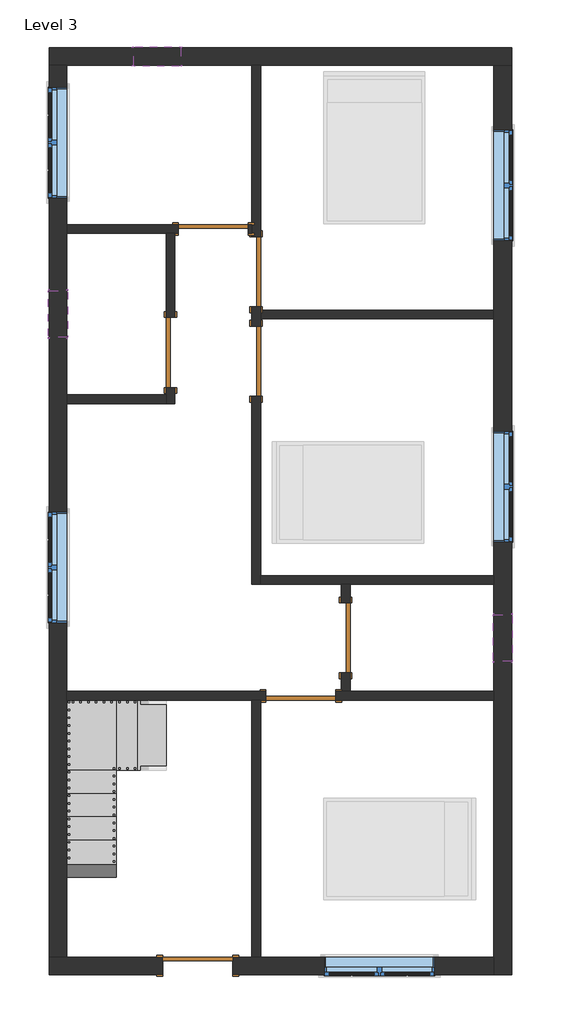
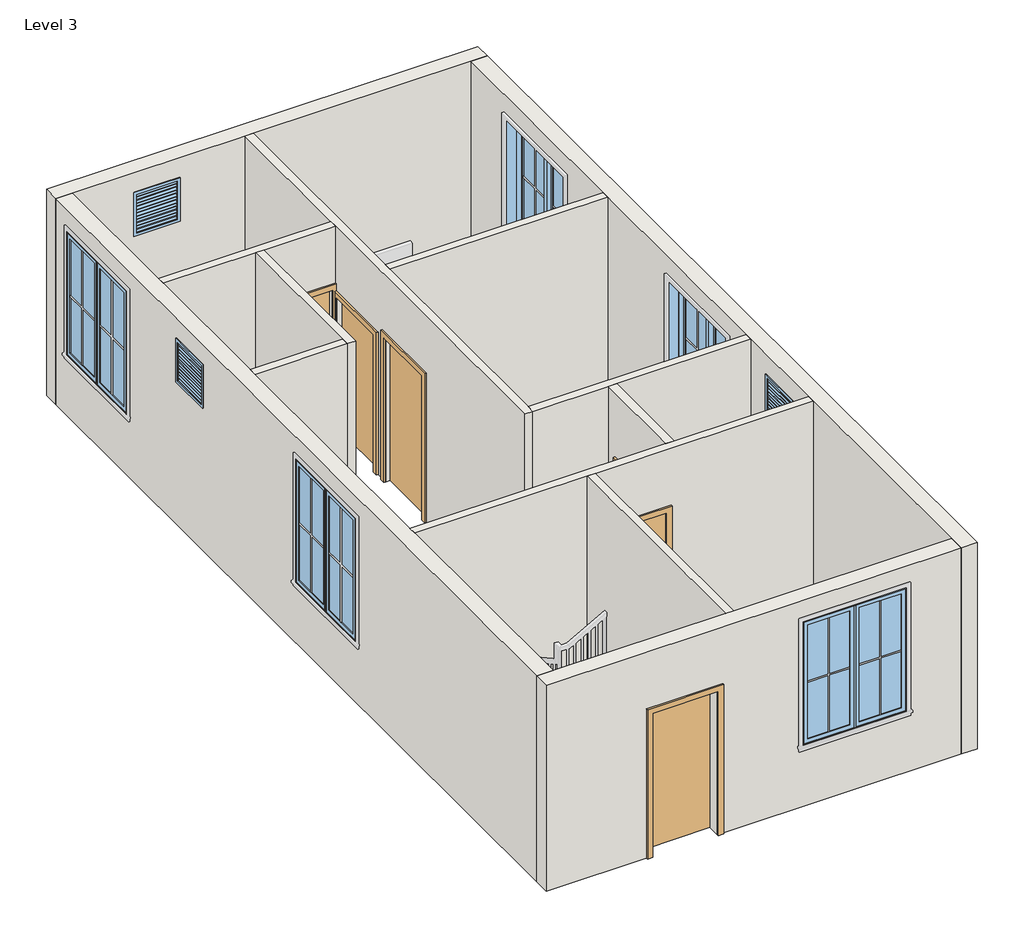
# One storey, part 1 of 2: 13 walls, 8 windows, 7 doors, 1 stair flight.
"""IFC4 building model written with IfcOpenShell, lengths in millimetres."""

from ifc_helpers import new_model, si_unit, frame, origin, place, context, project, spatial, polyline, outline, extrude, faceted_brep, transform, mapped, element, save
from components import door_5e62189b, door_17d80c48, door_e5f9f3c4, door_305aa2a5, door_0ca8825f, window_9ac97e1a, window_f2d8fef0

model = new_model("IFC4")

# Units and contexts
model_context = context("Model", 3, world=origin())
ifc_project = project(units=[si_unit("LENGTHUNIT", "METRE", prefix="MILLI")], contexts=[model_context])

# Site, building, storey
site = spatial("IfcSite", under=ifc_project)
building = spatial("IfcBuilding", under=site)
storey = spatial("IfcBuildingStorey", under=building, Name="Level 3", Elevation=3200.4)

# Doors
placement = place(None, origin())
door_shape = door_5e62189b(model_context)
element("IfcDoor", 1, ObjectType="Single-Flush : 36\" x 80\"", at=placement, inside=storey, context=model_context, shape_type="MappedRepresentation", body=[
    mapped(door_shape, transform((-2690.3389285, 2204.6069249, 3200.4), x_axis=(0.0, -1.0, 0.0), y_axis=(1.0, 0.0, 0.0), z_axis=(0.0, 0.0, 1.0))),
])
element("IfcDoor", 2, ObjectType="Single-Flush : 36\" x 80\"", at=placement, inside=storey, context=model_context, shape_type="MappedRepresentation", body=[
    mapped(door_shape, transform((-404.3389285, -1522.8430751, 3200.4), x_axis=(0.0, 1.0, 0.0), y_axis=(-1.0, 0.0, 0.0), z_axis=(0.0, 0.0, 1.0))),
])
door_2_shape = door_17d80c48(model_context)
element("IfcDoor", 3, ObjectType="Single-Flush : 36\" x 80\"", at=placement, inside=storey, context=model_context, shape_type="MappedRepresentation", body=[
    mapped(door_2_shape, transform((-1572.7389285, 3258.7069249, 3200.4), x_axis=(0.0, -1.0, 0.0), y_axis=(1.0, 0.0, 0.0), z_axis=(0.0, 0.0, 1.0))),
])
door_3_shape = door_e5f9f3c4(model_context)
element("IfcDoor", 4, ObjectType="Single-Flush : 36\" x 84\"", at=placement, inside=storey, context=model_context, shape_type="MappedRepresentation", body=[
    mapped(door_3_shape, transform((-2131.5389285, 3817.5069249, 3200.4), x_axis=(1.0, 0.0, 0.0), y_axis=(0.0, 1.0, 0.0), z_axis=(0.0, 0.0, 1.0))),
])
element("IfcDoor", 5, ObjectType="Single-Flush : 36\" x 84\"", at=placement, inside=storey, context=model_context, shape_type="MappedRepresentation", body=[
    mapped(door_3_shape, transform((-988.5389285, -2278.4930751, 3200.4), x_axis=(-1.0, 0.0, 0.0), y_axis=(0.0, -1.0, 0.0), z_axis=(0.0, 0.0, 1.0))),
])
door_4_shape = door_305aa2a5(model_context)
element("IfcDoor", 6, ObjectType="Single-Flush : 36\" x 84\"", at=placement, inside=storey, context=model_context, shape_type="MappedRepresentation", body=[
    mapped(door_4_shape, transform((-1572.7389285, 2090.3069249, 3200.4), x_axis=(0.0, 1.0, 0.0), y_axis=(-1.0, 0.0, 0.0), z_axis=(0.0, 0.0, 1.0))),
])
door_5_shape = door_0ca8825f(model_context)
element("IfcDoor", 7, ObjectType="Single-Flush : 36\" x 84\"", at=placement, inside=storey, context=model_context, shape_type="MappedRepresentation", body=[
    mapped(door_5_shape, transform((-2334.7389285, -5802.7430751, 3200.4), x_axis=(1.0, 0.0, 0.0), y_axis=(0.0, 1.0, 0.0), z_axis=(0.0, 0.0, 1.0))),
])

# Stair flight
element("IfcStairFlight", 8, ObjectType="3/4\" Nosing", at=placement, inside=storey, context=model_context, shape_type="Brep", body=[
    faceted_brep([(-2747.4889285, -3250.0430751, 3369.7333333), (-2747.4889285, -2335.6430751, 3369.7333333), (-3128.4889285, -2335.6430751, 3369.7333333), (-3128.4889285, -3250.0430751, 3369.7333333), (-3128.4889285, -3250.0430751, 3306.2333333), (-2754.6326785, -3250.0430751, 3306.2333333), (-2754.6326785, -2335.6430751, 3306.2333333), (-3128.4889285, -2335.6430751, 3306.2333333)], [[[0, 1, 2, 3]], [[0, 3, 4, 5]], [[2, 1, 6, 7]], [[1, 0, 5, 6]], [[4, 7, 6, 5]], [[7, 4, 3, 2]]]),
    faceted_brep([(-3128.4889285, -3250.0430751, 3539.0666667), (-3128.4889285, -2335.6430751, 3539.0666667), (-3401.5389285, -2335.6430751, 3539.0666667), (-3401.5389285, -3250.0430751, 3539.0666667), (-3401.5389285, -3250.0430751, 3475.5666667), (-3135.6326785, -3250.0430751, 3475.5666667), (-3135.6326785, -2335.6430751, 3475.5666667), (-3401.5389285, -2335.6430751, 3475.5666667)], [[[0, 1, 2, 3]], [[0, 3, 4, 5]], [[2, 1, 6, 7]], [[1, 0, 5, 6]], [[4, 7, 6, 5]], [[7, 4, 3, 2]]]),
    faceted_brep([(-3401.5389285, -3269.0930751, 3708.4), (-3401.5389285, -3250.0430751, 3708.4), (-3401.5389285, -2335.6430751, 3708.4), (-4042.8889285, -2335.6430751, 3708.4), (-4042.8889285, -3269.0930751, 3708.4), (-3401.5389285, -3269.0930751, 3644.9), (-3401.5389285, -3250.0430751, 3644.9), (-3408.6826785, -3250.0430751, 3644.9), (-3408.6826785, -2335.6430751, 3644.9), (-4042.8889285, -2335.6430751, 3644.9), (-4042.8889285, -3269.0930751, 3644.9), (-3401.5389285, -3250.0430751, 3877.7333333), (-4042.8889285, -3250.0430751, 3877.7333333), (-4042.8889285, -3285.5502386, 3877.7333333), (-4042.8889285, -3573.8930751, 3877.7333333), (-3401.5389285, -3573.8930751, 3877.7333333), (-3401.5389285, -3285.5502386, 3877.7333333), (-3401.5389285, -3573.8930751, 3805.1200976), (-3401.5389285, -3285.5502386, 3644.9), (-4042.8889285, -3285.5502386, 3644.9), (-4042.8889285, -3573.8930751, 3805.1200976), (-3401.5389285, -3554.8430751, 4047.0666667), (-4042.8889285, -3554.8430751, 4047.0666667), (-4042.8889285, -3878.6930751, 4047.0666667), (-3401.5389285, -3878.6930751, 4047.0666667), (-3401.5389285, -3878.6930751, 3974.4847552), (-4042.8889285, -3878.6930751, 3974.4847552), (-3401.5389285, -3859.6430751, 4216.4), (-4042.8889285, -3859.6430751, 4216.4), (-4042.8889285, -4183.4930751, 4216.4), (-3401.5389285, -4183.4930751, 4216.4), (-3401.5389285, -4183.4930751, 4143.8494128), (-4042.8889285, -4183.4930751, 4143.8494128), (-3401.5389285, -4164.4430751, 4385.7333333), (-4042.8889285, -4164.4430751, 4385.7333333), (-4042.8889285, -4488.2930751, 4385.7333333), (-3401.5389285, -4488.2930751, 4385.7333333), (-3401.5389285, -4488.2930751, 4313.2140703), (-4042.8889285, -4488.2930751, 4313.2140703), (-3401.5389285, -4792.8112092, 4555.0666667), (-3401.5389285, -4469.2430751, 4555.0666667), (-4042.8889285, -4469.2430751, 4555.0666667), (-4042.8889285, -4792.8112092, 4555.0666667), (-3401.5389285, -4773.7612092, 4724.4), (-3401.5389285, -5114.0119996, 4724.4), (-3401.5389285, -5114.0119996, 4660.9), (-4042.8889285, -4792.8112092, 4482.4221068), (-4042.8889285, -4773.7612092, 4724.4), (-4042.8889285, -5114.0119996, 4724.4), (-4042.8889285, -5688.4430751, 4724.4), (-3401.5389285, -5688.4430751, 4724.4), (-4042.8889285, -5114.0119996, 4660.9), (-4042.8889285, -5688.4430751, 4660.9), (-3401.5389285, -5688.4430751, 4660.9)], [[[0, 1, 2, 3, 4]], [[1, 0, 5, 6]], [[7, 1, 6]], [[3, 2, 8, 9]], [[4, 3, 9, 10]], [[11, 12, 13, 14, 15, 16]], [[0, 11, 16, 15, 17, 18, 5]], [[12, 4, 10, 19, 20, 14, 13]], [[21, 22, 23, 24]], [[21, 24, 25, 17, 15]], [[23, 22, 14, 20, 26]], [[27, 28, 29, 30]], [[27, 30, 31, 25, 24]], [[29, 28, 23, 26, 32]], [[33, 34, 35, 36]], [[33, 36, 37, 31, 30]], [[35, 34, 29, 32, 38]], [[39, 40, 41, 42]], [[39, 43, 44, 45, 37, 36, 40]], [[42, 41, 35, 38, 46]], [[43, 47, 48, 49, 50, 44]], [[47, 42, 46, 51, 52, 49, 48]], [[50, 49, 52, 53]], [[2, 1, 7, 8]], [[0, 4, 12, 11]], [[15, 14, 22, 21]], [[24, 23, 28, 27]], [[30, 29, 34, 33]], [[36, 35, 41, 40]], [[39, 42, 47, 43]], [[18, 19, 10, 9, 8, 7, 6, 5]], [[19, 18, 17, 25, 31, 37, 45, 51, 46, 38, 32, 26, 20]], [[45, 53, 52, 51]], [[53, 45, 44, 50]]]),
    faceted_brep([(-3401.5389285, -4773.7612092, 4893.7333333), (-3401.5389285, -5688.4430751, 4893.7333333), (-3128.4889285, -5688.4430751, 4893.7333333), (-3128.4889285, -4773.7612092, 4893.7333333), (-3394.3951785, -4773.7612092, 4830.2333333), (-3128.4889285, -4773.7612092, 4830.2333333), (-3394.3951785, -5688.4430751, 4830.2333333), (-3128.4889285, -5688.4430751, 4830.2333333)], [[[0, 1, 2, 3]], [[4, 0, 3, 5]], [[2, 1, 6, 7]], [[1, 0, 4, 6]], [[5, 7, 6, 4]], [[7, 5, 3, 2]]]),
    faceted_brep([(-3128.4889285, -4773.7612092, 5063.0666667), (-3128.4889285, -5688.4430751, 5063.0666667), (-2793.6303845, -5688.4430751, 5063.0666667), (-2793.6303845, -4773.7612092, 5063.0666667), (-2793.6303845, -4773.7612092, 4999.5666667), (-3121.3451785, -4773.7612092, 4999.5666667), (-3121.3451785, -5688.4430751, 4999.5666667), (-2793.6303845, -5688.4430751, 4999.5666667)], [[[0, 1, 2, 3]], [[0, 3, 4, 5]], [[2, 1, 6, 7]], [[3, 2, 7, 4]], [[1, 0, 5, 6]], [[6, 5, 4, 7]]]),
])

# Walls
element("IfcWall", 9, ObjectType="WALL 4.5\"", at=placement, inside=storey, context=model_context, shape_type="Brep", body=[
    faceted_brep([(-1629.8889285, 2801.5069249, 5232.4), (-1629.8889285, 2801.5069249, 3200.4), (-1629.8889285, 2547.5069249, 3200.4), (-1629.8889285, 2547.5069249, 5334.0), (-1629.8889285, 1633.1069249, 5334.0), (-1629.8889285, 1633.1069249, 3200.4), (-1629.8889285, -824.3430751, 3200.4), (-1629.8889285, -824.3430751, 6248.4), (-1629.8889285, 3760.3569249, 6248.4), (-1629.8889285, 3874.6569249, 6248.4), (-1629.8889285, 5957.4569249, 6248.4), (-1629.8889285, 5957.4569249, 3200.4), (-1629.8889285, 3874.6569249, 3200.4), (-1629.8889285, 3760.3569249, 3200.4), (-1629.8889285, 3715.9069249, 3200.4), (-1629.8889285, 3715.9069249, 5232.4), (-1515.5889285, 2547.5069249, 3200.4), (-1515.5889285, 2642.7569249, 3200.4), (-1515.5889285, 2757.0569249, 3200.4), (-1515.5889285, 2801.5069249, 3200.4), (-1515.5889285, 2801.5069249, 5232.4), (-1515.5889285, 3715.9069249, 5232.4), (-1515.5889285, 3715.9069249, 3200.4), (-1515.5889285, 5957.4569249, 3200.4), (-1515.5889285, 5957.4569249, 6248.4), (-1515.5889285, 2757.0569249, 6248.4), (-1515.5889285, 2642.7569249, 6248.4), (-1515.5889285, -710.0430751, 6248.4), (-1515.5889285, -824.3430751, 6248.4), (-1515.5889285, -824.3430751, 3200.4), (-1515.5889285, -710.0430751, 3200.4), (-1515.5889285, 1633.1069249, 3200.4), (-1515.5889285, 1633.1069249, 5334.0), (-1515.5889285, 2547.5069249, 5334.0)], [[[0, 1, 2, 3, 4, 5, 6, 7, 8, 9, 10, 11, 12, 13, 14, 15]], [[16, 17, 18, 19, 20, 21, 22, 23, 24, 25, 26, 27, 28, 29, 30, 31, 32, 33]], [[31, 30, 29, 6, 5]], [[2, 1, 19, 18, 17, 16]], [[14, 13, 12, 11, 23, 22]], [[11, 10, 24, 23]], [[3, 2, 16, 33]], [[4, 3, 33, 32]], [[5, 4, 32, 31]], [[20, 19, 1, 0]], [[21, 20, 0, 15]], [[22, 21, 15, 14]], [[10, 9, 8, 7, 28, 27, 26, 25, 24]], [[7, 6, 29, 28]]]),
])
element("IfcWall", 10, ObjectType="WALL 4.5\"", at=placement, inside=storey, context=model_context, shape_type="Brep", body=[
    faceted_brep([(1532.4110715, -710.0430751, 3200.4), (-1515.5889285, -710.0430751, 3200.4), (-1515.5889285, -710.0430751, 6248.4), (1532.4110715, -710.0430751, 6248.4), (1532.4110715, -824.3430751, 3200.4), (1532.4110715, -824.3430751, 6248.4), (-347.1889285, -824.3430751, 6248.4), (-461.4889285, -824.3430751, 6248.4), (-1515.5889285, -824.3430751, 6248.4), (-1515.5889285, -824.3430751, 3200.4), (-461.4889285, -824.3430751, 3200.4), (-347.1889285, -824.3430751, 3200.4)], [[[0, 1, 2, 3]], [[4, 5, 6, 7, 8, 9, 10, 11]], [[1, 0, 4, 11, 10, 9]], [[0, 3, 5, 4]], [[3, 2, 8, 7, 6, 5]], [[2, 1, 9, 8]]]),
])
element("IfcWall", 11, ObjectType="WALL 4.5\"", at=placement, inside=storey, context=model_context, shape_type="SweptSolid", body=[
    extrude(outline(polyline([(-1515.5889285, 2757.0569249), (1532.4110715, 2757.0569249), (1532.4110715, 2642.7569249), (-1515.5889285, 2642.7569249), (-1515.5889285, 2757.0569249)])), frame((0.0, 0.0, 3200.4), z_axis=(0.0, 0.0, 1.0), x_axis=(1.0, 0.0, 0.0)), (0.0, 0.0, 1.0), 3048.0),
])
element("IfcWall", 12, ObjectType="WALL 4.5\"", at=placement, inside=storey, context=model_context, shape_type="Brep", body=[
    faceted_brep([(-1674.3389285, 3760.3569249, 5334.0), (-1674.3389285, 3760.3569249, 3200.4), (-1629.8889285, 3760.3569249, 3200.4), (-1629.8889285, 3760.3569249, 6248.4), (-2633.1889285, 3760.3569249, 6248.4), (-2747.4889285, 3760.3569249, 6248.4), (-4042.8889285, 3760.3569249, 6248.4), (-4042.8889285, 3760.3569249, 3200.4), (-2747.4889285, 3760.3569249, 3200.4), (-2633.1889285, 3760.3569249, 3200.4), (-2588.7389285, 3760.3569249, 3200.4), (-2588.7389285, 3760.3569249, 5334.0), (-1629.8889285, 3874.6569249, 3200.4), (-1674.3389285, 3874.6569249, 3200.4), (-1674.3389285, 3874.6569249, 5334.0), (-2588.7389285, 3874.6569249, 5334.0), (-2588.7389285, 3874.6569249, 3200.4), (-4042.8889285, 3874.6569249, 3200.4), (-4042.8889285, 3874.6569249, 6248.4), (-1629.8889285, 3874.6569249, 6248.4)], [[[0, 1, 2, 3, 4, 5, 6, 7, 8, 9, 10, 11]], [[12, 13, 14, 15, 16, 17, 18, 19]], [[2, 1, 13, 12]], [[10, 9, 8, 7, 17, 16]], [[7, 6, 18, 17]], [[3, 2, 12, 19]], [[14, 13, 1, 0]], [[15, 14, 0, 11]], [[16, 15, 11, 10]], [[6, 5, 4, 3, 19, 18]]]),
])
element("IfcWall", 13, ObjectType="WALL 4.5\"", at=placement, inside=storey, context=model_context, shape_type="Brep", body=[
    faceted_brep([(-2747.4889285, 1747.4069249, 5232.4), (-2747.4889285, 1747.4069249, 3200.4), (-2747.4889285, 1652.1569249, 3200.4), (-2747.4889285, 1537.8569249, 3200.4), (-2747.4889285, 1537.8569249, 6248.4), (-2747.4889285, 1652.1569249, 6248.4), (-2747.4889285, 3760.3569249, 6248.4), (-2747.4889285, 3760.3569249, 3200.4), (-2747.4889285, 2661.8069249, 3200.4), (-2747.4889285, 2661.8069249, 5232.4), (-2633.1889285, 1537.8569249, 3200.4), (-2633.1889285, 1747.4069249, 3200.4), (-2633.1889285, 1747.4069249, 5232.4), (-2633.1889285, 2661.8069249, 5232.4), (-2633.1889285, 2661.8069249, 3200.4), (-2633.1889285, 3760.3569249, 3200.4), (-2633.1889285, 3760.3569249, 6248.4), (-2633.1889285, 1537.8569249, 6248.4)], [[[0, 1, 2, 3, 4, 5, 6, 7, 8, 9]], [[10, 11, 12, 13, 14, 15, 16, 17]], [[8, 7, 15, 14]], [[3, 2, 1, 11, 10]], [[7, 6, 16, 15]], [[4, 3, 10, 17]], [[12, 11, 1, 0]], [[13, 12, 0, 9]], [[14, 13, 9, 8]], [[6, 5, 4, 17, 16]]]),
])
element("IfcWall", 14, ObjectType="WALL 4.5\"", at=placement, inside=storey, context=model_context, shape_type="SweptSolid", body=[
    extrude(outline(polyline([(-4042.8889285, 1652.1569249), (-2747.4889285, 1652.1569249), (-2747.4889285, 1537.8569249), (-4042.8889285, 1537.8569249), (-4042.8889285, 1652.1569249)])), frame((0.0, 0.0, 3200.4), z_axis=(0.0, 0.0, 1.0), x_axis=(1.0, 0.0, 0.0)), (0.0, 0.0, 1.0), 3048.0),
])
element("IfcWall", 15, ObjectType="WALL 4.5\"", at=placement, inside=storey, context=model_context, shape_type="Brep", body=[
    faceted_brep([(-4042.8889285, -2335.6430751, 3200.4), (-1629.8889285, -2335.6430751, 3200.4), (-1515.5889285, -2335.6430751, 3200.4), (-1445.7389285, -2335.6430751, 3200.4), (-1445.7389285, -2335.6430751, 5334.0), (-531.3389285, -2335.6430751, 5334.0), (-531.3389285, -2335.6430751, 3200.4), (1532.4110715, -2335.6430751, 3200.4), (1532.4110715, -2335.6430751, 6248.4), (-1515.5889285, -2335.6430751, 6248.4), (-1629.8889285, -2335.6430751, 6248.4), (-4042.8889285, -2335.6430751, 6248.4), (-1445.7389285, -2221.3430751, 5334.0), (-1445.7389285, -2221.3430751, 3200.4), (-4042.8889285, -2221.3430751, 3200.4), (-4042.8889285, -2221.3430751, 6248.4), (-461.4889285, -2221.3430751, 6248.4), (-347.1889285, -2221.3430751, 6248.4), (1532.4110715, -2221.3430751, 6248.4), (1532.4110715, -2221.3430751, 3200.4), (-347.1889285, -2221.3430751, 3200.4), (-461.4889285, -2221.3430751, 3200.4), (-531.3389285, -2221.3430751, 3200.4), (-531.3389285, -2221.3430751, 5334.0)], [[[0, 1, 2, 3, 4, 5, 6, 7, 8, 9, 10, 11]], [[12, 13, 14, 15, 16, 17, 18, 19, 20, 21, 22, 23]], [[14, 13, 3, 2, 1, 0]], [[22, 21, 20, 19, 7, 6]], [[8, 7, 19, 18]], [[0, 11, 15, 14]], [[4, 3, 13, 12]], [[5, 4, 12, 23]], [[6, 5, 23, 22]], [[11, 10, 9, 8, 18, 17, 16, 15]]]),
])
element("IfcWall", 16, ObjectType="WALL 4.5\"", at=placement, inside=storey, context=model_context, shape_type="SweptSolid", body=[
    extrude(outline(polyline([(-824.3430751, 3200.4), (-1065.6430751, 3200.4), (-1065.6430751, 5232.4), (-1980.0430751, 5232.4), (-1980.0430751, 3200.4), (-2221.3430751, 3200.4), (-2221.3430751, 6248.4), (-824.3430751, 6248.4), (-824.3430751, 3200.4)])), frame((-461.4889285, 0.0, 0.0), z_axis=(1.0, 0.0, 0.0), x_axis=(0.0, 1.0, 0.0)), (0.0, 0.0, 1.0), 114.3),
])
element("IfcWall", 17, ObjectType="WALL 4.5\"", at=placement, inside=storey, context=model_context, shape_type="SweptSolid", body=[
    extrude(outline(polyline([(-1629.8889285, -5688.4430751), (-1629.8889285, -2335.6430751), (-1515.5889285, -2335.6430751), (-1515.5889285, -5688.4430751), (-1629.8889285, -5688.4430751)])), frame((0.0, 0.0, 3200.4), z_axis=(0.0, 0.0, 1.0), x_axis=(1.0, 0.0, 0.0)), (0.0, 0.0, 1.0), 3048.0),
])
element("IfcWall", 18, ObjectType="WALL 9\"", at=placement, inside=storey, context=model_context, shape_type="Brep", body=[
    faceted_brep([(-4271.4889285, 5957.4569249, 3200.4), (-4042.8889285, 5957.4569249, 3200.4), (-1629.8889285, 5957.4569249, 3200.4), (-1515.5889285, 5957.4569249, 3200.4), (1532.4110715, 5957.4569249, 3200.4), (1761.0110715, 5957.4569249, 3200.4), (1761.0110715, 5957.4569249, 6248.4), (1532.4110715, 5957.4569249, 6248.4), (-1515.5889285, 5957.4569249, 6248.4), (-1629.8889285, 5957.4569249, 6248.4), (-4042.8889285, 5957.4569249, 6248.4), (-4271.4889285, 5957.4569249, 6248.4), (-2560.1639285, 5957.4569249, 5943.6), (-2560.1639285, 5957.4569249, 5334.0), (-3169.7639285, 5957.4569249, 5334.0), (-3169.7639285, 5957.4569249, 5943.6), (-4271.4889285, 6186.0569249, 3200.4), (-4271.4889285, 6186.0569249, 6248.4), (1761.0110715, 6186.0569249, 6248.4), (1761.0110715, 6186.0569249, 3200.4), (-2560.1639285, 6186.0569249, 5943.6), (-3169.7639285, 6186.0569249, 5943.6), (-3169.7639285, 6186.0569249, 5334.0), (-2560.1639285, 6186.0569249, 5334.0)], [[[0, 1, 2, 3, 4, 5, 6, 7, 8, 9, 10, 11], [12, 13, 14, 15]], [[16, 17, 18, 19], [20, 21, 22, 23]], [[5, 4, 3, 2, 1, 0, 16, 19]], [[6, 5, 19, 18]], [[0, 11, 17, 16]], [[13, 12, 20, 23]], [[14, 13, 23, 22]], [[15, 14, 22, 21]], [[12, 15, 21, 20]], [[11, 10, 9, 8, 7, 6, 18, 17]]]),
])
element("IfcWall", 19, ObjectType="WALL 9\"", at=placement, inside=storey, context=model_context, shape_type="Brep", body=[
    faceted_brep([(1532.4110715, 5957.4569249, 3200.4), (1532.4110715, 2757.0569249, 3200.4), (1532.4110715, 2642.7569249, 3200.4), (1532.4110715, -710.0430751, 3200.4), (1532.4110715, -824.3430751, 3200.4), (1532.4110715, -2221.3430751, 3200.4), (1532.4110715, -2335.6430751, 3200.4), (1532.4110715, -5688.4430751, 3200.4), (1532.4110715, -5917.0430751, 3200.4), (1532.4110715, -5917.0430751, 6248.4), (1532.4110715, -5688.4430751, 6248.4), (1532.4110715, -2335.6430751, 6248.4), (1532.4110715, -2221.3430751, 6248.4), (1532.4110715, -824.3430751, 6248.4), (1532.4110715, -710.0430751, 6248.4), (1532.4110715, 2642.7569249, 6248.4), (1532.4110715, 2757.0569249, 6248.4), (1532.4110715, 5957.4569249, 6248.4), (1532.4110715, 3661.9319249, 5943.6), (1532.4110715, 3661.9319249, 4114.8), (1532.4110715, 5109.7319249, 4114.8), (1532.4110715, 5109.7319249, 5943.6), (1532.4110715, -271.8930751, 5943.6), (1532.4110715, -271.8930751, 4114.8), (1532.4110715, 1175.9069249, 4114.8), (1532.4110715, 1175.9069249, 5943.6), (1532.4110715, -1827.6430751, 5943.6), (1532.4110715, -1827.6430751, 5334.0), (1532.4110715, -1218.0430751, 5334.0), (1532.4110715, -1218.0430751, 5943.6), (1761.0110715, 5957.4569249, 3200.4), (1761.0110715, 5957.4569249, 6248.4), (1761.0110715, -5917.0430751, 6248.4), (1761.0110715, -5917.0430751, 3200.4), (1761.0110715, 3661.9319249, 5943.6), (1761.0110715, 5109.7319249, 5943.6), (1761.0110715, 5109.7319249, 4114.8), (1761.0110715, 3661.9319249, 4114.8), (1761.0110715, -271.8930751, 5943.6), (1761.0110715, 1175.9069249, 5943.6), (1761.0110715, 1175.9069249, 4114.8), (1761.0110715, -271.8930751, 4114.8), (1761.0110715, -1827.6430751, 5943.6), (1761.0110715, -1218.0430751, 5943.6), (1761.0110715, -1218.0430751, 5334.0), (1761.0110715, -1827.6430751, 5334.0)], [[[0, 1, 2, 3, 4, 5, 6, 7, 8, 9, 10, 11, 12, 13, 14, 15, 16, 17], [18, 19, 20, 21], [22, 23, 24, 25], [26, 27, 28, 29]], [[30, 31, 32, 33], [34, 35, 36, 37], [38, 39, 40, 41], [42, 43, 44, 45]], [[8, 7, 6, 5, 4, 3, 2, 1, 0, 30, 33]], [[0, 17, 31, 30]], [[9, 8, 33, 32]], [[19, 18, 34, 37]], [[20, 19, 37, 36]], [[21, 20, 36, 35]], [[18, 21, 35, 34]], [[23, 22, 38, 41]], [[24, 23, 41, 40]], [[25, 24, 40, 39]], [[22, 25, 39, 38]], [[27, 26, 42, 45]], [[28, 27, 45, 44]], [[29, 28, 44, 43]], [[26, 29, 43, 42]], [[17, 16, 15, 14, 13, 12, 11, 10, 9, 32, 31]]]),
])
element("IfcWall", 20, ObjectType="WALL 9\"", at=placement, inside=storey, context=model_context, shape_type="Brep", body=[
    faceted_brep([(1532.4110715, -5688.4430751, 3200.4), (-1515.5889285, -5688.4430751, 3200.4), (-1629.8889285, -5688.4430751, 3200.4), (-1877.5389285, -5688.4430751, 3200.4), (-1877.5389285, -5688.4430751, 5334.0), (-2791.9389285, -5688.4430751, 5334.0), (-2791.9389285, -5688.4430751, 3200.4), (-4042.8889285, -5688.4430751, 3200.4), (-4271.4889285, -5688.4430751, 3200.4), (-4271.4889285, -5688.4430751, 6248.4), (-4042.8889285, -5688.4430751, 6248.4), (-1629.8889285, -5688.4430751, 6248.4), (-1515.5889285, -5688.4430751, 6248.4), (1532.4110715, -5688.4430751, 6248.4), (-686.9139285, -5688.4430751, 5943.6), (-686.9139285, -5688.4430751, 4114.8), (760.8860715, -5688.4430751, 4114.8), (760.8860715, -5688.4430751, 5943.6), (-1877.5389285, -5917.0430751, 5334.0), (-1877.5389285, -5917.0430751, 3200.4), (1532.4110715, -5917.0430751, 3200.4), (1532.4110715, -5917.0430751, 6248.4), (-4271.4889285, -5917.0430751, 6248.4), (-4271.4889285, -5917.0430751, 3200.4), (-2791.9389285, -5917.0430751, 3200.4), (-2791.9389285, -5917.0430751, 5334.0), (-686.9139285, -5917.0430751, 5943.6), (760.8860715, -5917.0430751, 5943.6), (760.8860715, -5917.0430751, 4114.8), (-686.9139285, -5917.0430751, 4114.8)], [[[0, 1, 2, 3, 4, 5, 6, 7, 8, 9, 10, 11, 12, 13], [14, 15, 16, 17]], [[18, 19, 20, 21, 22, 23, 24, 25], [26, 27, 28, 29]], [[24, 23, 8, 7, 6]], [[20, 19, 3, 2, 1, 0]], [[0, 13, 21, 20]], [[9, 8, 23, 22]], [[15, 14, 26, 29]], [[16, 15, 29, 28]], [[17, 16, 28, 27]], [[14, 17, 27, 26]], [[4, 3, 19, 18]], [[5, 4, 18, 25]], [[6, 5, 25, 24]], [[13, 12, 11, 10, 9, 22, 21]]]),
])
element("IfcWall", 21, ObjectType="WALL 9\"", at=placement, inside=storey, context=model_context, shape_type="Brep", body=[
    faceted_brep([(-4042.8889285, -5688.4430751, 3200.4), (-4042.8889285, -2335.6430751, 3200.4), (-4042.8889285, -2221.3430751, 3200.4), (-4042.8889285, 1537.8569249, 3200.4), (-4042.8889285, 1652.1569249, 3200.4), (-4042.8889285, 3760.3569249, 3200.4), (-4042.8889285, 3874.6569249, 3200.4), (-4042.8889285, 5957.4569249, 3200.4), (-4042.8889285, 5957.4569249, 6248.4), (-4042.8889285, 3874.6569249, 6248.4), (-4042.8889285, 3760.3569249, 6248.4), (-4042.8889285, 1652.1569249, 6248.4), (-4042.8889285, 1537.8569249, 6248.4), (-4042.8889285, -2221.3430751, 6248.4), (-4042.8889285, -2335.6430751, 6248.4), (-4042.8889285, -5688.4430751, 6248.4), (-4042.8889285, 5668.5319249, 5943.6), (-4042.8889285, 5668.5319249, 4114.8), (-4042.8889285, 4220.7319249, 4114.8), (-4042.8889285, 4220.7319249, 5943.6), (-4042.8889285, 121.8069249, 5943.6), (-4042.8889285, 121.8069249, 4114.8), (-4042.8889285, -1325.9930751, 4114.8), (-4042.8889285, -1325.9930751, 5943.6), (-4042.8889285, 2401.4569249, 5943.6), (-4042.8889285, 3011.0569249, 5943.6), (-4042.8889285, 3011.0569249, 5334.0), (-4042.8889285, 2401.4569249, 5334.0), (-4271.4889285, -5688.4430751, 3200.4), (-4271.4889285, -5688.4430751, 6248.4), (-4271.4889285, 5957.4569249, 6248.4), (-4271.4889285, 5957.4569249, 3200.4), (-4271.4889285, 5668.5319249, 5943.6), (-4271.4889285, 4220.7319249, 5943.6), (-4271.4889285, 4220.7319249, 4114.8), (-4271.4889285, 5668.5319249, 4114.8), (-4271.4889285, 121.8069249, 5943.6), (-4271.4889285, -1325.9930751, 5943.6), (-4271.4889285, -1325.9930751, 4114.8), (-4271.4889285, 121.8069249, 4114.8), (-4271.4889285, 2401.4569249, 5943.6), (-4271.4889285, 2401.4569249, 5334.0), (-4271.4889285, 3011.0569249, 5334.0), (-4271.4889285, 3011.0569249, 5943.6)], [[[0, 1, 2, 3, 4, 5, 6, 7, 8, 9, 10, 11, 12, 13, 14, 15], [16, 17, 18, 19], [20, 21, 22, 23], [24, 25, 26, 27]], [[28, 29, 30, 31], [32, 33, 34, 35], [36, 37, 38, 39], [40, 41, 42, 43]], [[7, 6, 5, 4, 3, 2, 1, 0, 28, 31]], [[0, 15, 29, 28]], [[8, 7, 31, 30]], [[17, 16, 32, 35]], [[18, 17, 35, 34]], [[19, 18, 34, 33]], [[16, 19, 33, 32]], [[21, 20, 36, 39]], [[22, 21, 39, 38]], [[23, 22, 38, 37]], [[20, 23, 37, 36]], [[41, 40, 24, 27]], [[42, 41, 27, 26]], [[43, 42, 26, 25]], [[40, 43, 25, 24]], [[15, 14, 13, 12, 11, 10, 9, 8, 30, 29]]]),
])

# Windows
window_shape = window_9ac97e1a(model_context)
element("IfcWindow", 22, ObjectType="Window-Casement-Double : 57\" x 72\"", at=placement, inside=storey, context=model_context, shape_type="MappedRepresentation", body=[
    mapped(window_shape, transform((-4157.1889285, 4944.6319249, 3200.4), x_axis=(0.0, 1.0, 0.0), y_axis=(-1.0, 0.0, 0.0), z_axis=(0.0, 0.0, 1.0))),
])
element("IfcWindow", 23, ObjectType="Window-Casement-Double : 57\" x 72\"", at=placement, inside=storey, context=model_context, shape_type="MappedRepresentation", body=[
    mapped(window_shape, transform((1646.7110715, 4385.8319249, 3200.4), x_axis=(0.0, -1.0, 0.0), y_axis=(1.0, 0.0, 0.0), z_axis=(0.0, 0.0, 1.0))),
])
element("IfcWindow", 24, ObjectType="Window-Casement-Double : 57\" x 72\"", at=placement, inside=storey, context=model_context, shape_type="MappedRepresentation", body=[
    mapped(window_shape, transform((-4157.1889285, -602.0930751, 3200.4), x_axis=(0.0, 1.0, 0.0), y_axis=(-1.0, 0.0, 0.0), z_axis=(0.0, 0.0, 1.0))),
])
element("IfcWindow", 25, ObjectType="Window-Casement-Double : 57\" x 72\"", at=placement, inside=storey, context=model_context, shape_type="MappedRepresentation", body=[
    mapped(window_shape, transform((1646.7110715, 452.0069249, 3200.4), x_axis=(0.0, -1.0, 0.0), y_axis=(1.0, 0.0, 0.0), z_axis=(0.0, 0.0, 1.0))),
])
element("IfcWindow", 26, ObjectType="Window-Casement-Double : 57\" x 72\"", at=placement, inside=storey, context=model_context, shape_type="MappedRepresentation", body=[
    mapped(window_shape, transform((36.9860715, -5802.7430751, 3200.4), x_axis=(-1.0, 0.0, 0.0), y_axis=(0.0, -1.0, 0.0), z_axis=(0.0, 0.0, 1.0))),
])
window_2_shape = window_f2d8fef0(model_context)
element("IfcWindow", 27, ObjectType="Window-Louvers : 24\" x 24\"", at=placement, inside=storey, context=model_context, shape_type="MappedRepresentation", body=[
    mapped(window_2_shape, transform((-2864.9639285, 6065.4069249, 4419.6), x_axis=(-1.0, 0.0, 0.0), y_axis=(0.0, -1.0, 0.0), z_axis=(0.0, 0.0, 1.0))),
])
element("IfcWindow", 28, ObjectType="Window-Louvers : 24\" x 24\"", at=placement, inside=storey, context=model_context, shape_type="MappedRepresentation", body=[
    mapped(window_2_shape, transform((-4163.5389285, 2706.2569249, 4419.6), x_axis=(0.0, 1.0, 0.0), y_axis=(-1.0, 0.0, 0.0), z_axis=(0.0, 0.0, 1.0))),
])
element("IfcWindow", 29, ObjectType="Window-Louvers : 24\" x 24\"", at=placement, inside=storey, context=model_context, shape_type="MappedRepresentation", body=[
    mapped(window_2_shape, transform((1640.3610715, -1522.8430751, 4419.6), x_axis=(0.0, 1.0, 0.0), y_axis=(-1.0, 0.0, 0.0), z_axis=(0.0, 0.0, 1.0))),
])

save(model, "model.ifc")

# Revit data of these elements
# Type "Single-Flush : 36\" x 80\""
#   Type Mark = "6"
#   Construction Type Id = "MDOOR"
#   Assembly Code = "C1020"
#   Analytic Construction = "Metal"
#   Thickness = 0' - 2"
#   Heat Transfer Coefficient (U) = 0.651978 BTU/(h·ft²·°F)
#   Height = 6' - 8"
#   Trim Projection Ext = 0' - 1"
#   Trim Projection Int = 0' - 1"
#   Trim Width = 0' - 3"
#   Width = 3' - 0"
#   Define Thermal Properties by = 1
#   Define Thermal Properties by = 1
#   Door Material = Door - Panel
#   Frame Material = Door - Frame
#   Visual Light Transmittance = 0
#   Solar Heat Gain Coefficient = 0
#   Function = (empty or 0)
#   Wall Closure = (empty or 0)
# Type "Single-Flush : 36\" x 84\""
#   Type Mark = "1"
#   Construction Type Id = "MDOOR"
#   Assembly Code = "C1020"
#   Analytic Construction = "Metal"
#   Thickness = 0' - 2"
#   Heat Transfer Coefficient (U) = 0.651978 BTU/(h·ft²·°F)
#   Height = 7' - 0"
#   Trim Projection Ext = 0' - 1"
#   Trim Projection Int = 0' - 1"
#   Trim Width = 0' - 3"
#   Width = 3' - 0"
#   Define Thermal Properties by = 1
#   Define Thermal Properties by = 1
#   Door Material = Door - Panel
#   Frame Material = Door - Frame
#   Visual Light Transmittance = 0
#   Solar Heat Gain Coefficient = 0
#   Function = (empty or 0)
#   Wall Closure = (empty or 0)
# Type "WALL 4.5\""
#   Assembly Code = "B2010"
#   Layers, outside or top first: 0' - 4 1/2" no material (function 1)
# Type "WALL 9\""
#   Assembly Code = "B2010"
#   Layers, outside or top first: 0' - 9" no material (function 1)
# Type "Window-Casement-Double : 57\" x 72\""
#   Type Mark = "17"
#   Fire Rating = "0.5h"
#   Assembly Code = "B2020100"
#   Analytic Construction = "Double glazing - domestic"
#   Frame Extension [instance default] = 0' - 0 1/4"
#   Window Inset [instance default] = 0' - 0"
#   Wall Thickness [instance default] = 0' - 6"
#   Interior Wall Closure [instance default] = 0' - 2 1/4"
#   Half Width = 2' - 4 1/2"
#   Visual Light Transmittance = 0.81
#   Thermal Resistance (R) = 1.8146 (h·ft²·°F)/BTU
#   Solar Heat Gain Coefficient = 0.76
#   Rough Width = 4' - 9 1/2"
#   Rough Height = 6' - 0 1/2"
#   Height = 6' - 0"
#   Heat Transfer Coefficient (U) = 0.5511 BTU/(h·ft²·°F)
#   Exterior Wall Closure [instance default] = 0' - 1 1/4"
#   Extension Jamb [instance default] = 0' - 2 1/4"
#   Default Sill Height = 3' - 0"
#   Width = 4' - 9"
#   Define Thermal Properties by = 0
#   Muntin Visibility = yes
#   Interior Trim Visibility [instance default] = yes
#   Exterior Trim Visibility [instance default] = yes
#   Extension Jamb Visibility [instance default] = yes
#   Interior Trim Material = Wood - Stained
#   Muntin Pattern = Muntin Pattern_2x2 : Muntin Pattern_2x2
#   Interior Trim = Trim-Window-Interior-Flat : Picture Frame
#   Interior Frame Material = Wood - Stained
#   Glass Panel Material = Glass
#   Exterior Trim Material = Clad - White
#   Exterior Trim = Trim-Window-Exterior-Flat : with Sill
#   Exterior Frame Material = Clad - White
#   Wall Closure = (empty or 0)
# Type "Window-Louvers : 24\" x 24\""
#   Type Mark = "18"
#   Construction Type Id = "GSP4R"
#   Assembly Code = "B20"
#   Analytic Construction = "1/8 in Pilkington single glazing"
#   Visual Light Transmittance = 0.9
#   Thermal Resistance (R) = 1.53941 (h·ft²·°F)/BTU
#   Solar Heat Gain Coefficient = 0.78
#   Max Height = 1' - 11.74264"
#   Height = 2' - 0"
#   Heat Transfer Coefficient (U) = 0.6496 BTU/(h·ft²·°F)
#   Blade Width [instance default] = 1' - 10 1/2"
#   Blade Vertical Thickness = 0' - 0.35355"
#   Blade Thickness = 0' - 0 1/4"
#   Blade Spacing = 0' - 1 1/2"
#   Blade Height = 0' - 1.85355"
#   Blade Depth = 0' - 3"
#   Blade Angle = 45.00°
#   Default Sill Height = 3' - 0"
#   Trim Projection_Exterior = 0' - 0 1/2"
#   Trim Projection_Interior = 0' - 0 1/2"
#   Trim Width_Exterior = 0' - 1 1/2"
#   Trim Width_Interior = 0' - 1 1/2"
#   Width = 2' - 0"
#   Max Blade Count = 12
#   Define Thermal Properties by = 1
#   Blade Count = 12
#   Frame Material = Birch
#   Louver Material = Birch
#   Trim Exterior Material = Birch
#   Trim Interior Material = Birch
#   Wall Closure = (empty or 0)
# Elements 1, 2, 3 (IfcDoor, "Single-Flush : 36\" x 80\"")
#   Phase Created = New Construction
#   Materials on its faces: "Door - Frame", "Door - Panel"
# Elements 4, 5, 6, 7 (IfcDoor, "Single-Flush : 36\" x 84\"")
#   Phase Created = New Construction
#   Materials on its faces: "Door - Frame", "Door - Panel"
# Element 8 (IfcStairFlight, "3/4\" Nosing")
#   Phase Created = New Construction
#   Materials on its faces: "Concrete, Cast-in-Place gray"
# Elements 9, 10, 11, 12, 13, 14, 15, 16, 17 (IfcWall, "WALL 4.5\"")
#   Top Offset = 0' - 0"
#   Base Offset = 0' - 0"
#   Unconnected Height = 10' - 0"
#   wall height = 10' - 0"
#   Phase Created = New Construction
#   Base Constraint = Level 3
#   Materials on its faces: "Default Wall"
# Elements 18, 19, 20, 21 (IfcWall, "WALL 9\"")
#   Top Offset = 0' - 0"
#   Base Offset = 0' - 0"
#   Unconnected Height = 10' - 0"
#   wall height = 10' - 0"
#   Phase Created = New Construction
#   Base Constraint = Level 3
#   Materials on its faces: "Default Wall", "Copper"
# Element 22 (IfcWindow, "Window-Casement-Double : 57\" x 72\"")
#   Mark = "9"
#   Window Inset = 0' - 0"
#   Interior Wall Closure = 0' - 2 1/4"
#   Frame Extension = 0' - 0 1/4"
#   Exterior Wall Closure = 0' - 1 1/4"
#   Interior Trim Visibility = yes
#   Exterior Trim Visibility = yes
#   Phase Created = New Construction
#   Materials on its faces: "Wood - Stained", "Glass", "Clad - White"
# Element 23 (IfcWindow, "Window-Casement-Double : 57\" x 72\"")
#   Mark = "10"
#   Window Inset = 0' - 0"
#   Interior Wall Closure = 0' - 2 1/4"
#   Frame Extension = 0' - 0 1/4"
#   Exterior Wall Closure = 0' - 1 1/4"
#   Interior Trim Visibility = yes
#   Exterior Trim Visibility = yes
#   Phase Created = New Construction
#   Materials on its faces: "Wood - Stained", "Glass", "Clad - White"
# Element 24 (IfcWindow, "Window-Casement-Double : 57\" x 72\"")
#   Mark = "11"
#   Window Inset = 0' - 0"
#   Interior Wall Closure = 0' - 2 1/4"
#   Frame Extension = 0' - 0 1/4"
#   Exterior Wall Closure = 0' - 1 1/4"
#   Interior Trim Visibility = yes
#   Exterior Trim Visibility = yes
#   Phase Created = New Construction
#   Materials on its faces: "Wood - Stained", "Glass", "Clad - White"
# Element 25 (IfcWindow, "Window-Casement-Double : 57\" x 72\"")
#   Mark = "12"
#   Window Inset = 0' - 0"
#   Interior Wall Closure = 0' - 2 1/4"
#   Frame Extension = 0' - 0 1/4"
#   Exterior Wall Closure = 0' - 1 1/4"
#   Interior Trim Visibility = yes
#   Exterior Trim Visibility = yes
#   Phase Created = New Construction
#   Materials on its faces: "Wood - Stained", "Glass", "Clad - White"
# Element 26 (IfcWindow, "Window-Casement-Double : 57\" x 72\"")
#   Mark = "13"
#   Window Inset = 0' - 0"
#   Interior Wall Closure = 0' - 2 1/4"
#   Frame Extension = 0' - 0 1/4"
#   Exterior Wall Closure = 0' - 1 1/4"
#   Interior Trim Visibility = yes
#   Exterior Trim Visibility = yes
#   Phase Created = New Construction
#   Materials on its faces: "Wood - Stained", "Glass", "Clad - White"
# Element 27 (IfcWindow, "Window-Louvers : 24\" x 24\"")
#   Mark = "14"
#   Blade Width = 1' - 10 1/2"
#   Phase Created = New Construction
#   Materials on its faces: "Birch"
# Element 28 (IfcWindow, "Window-Louvers : 24\" x 24\"")
#   Mark = "15"
#   Blade Width = 1' - 10 1/2"
#   Phase Created = New Construction
#   Materials on its faces: "Birch"
# Element 29 (IfcWindow, "Window-Louvers : 24\" x 24\"")
#   Mark = "16"
#   Blade Width = 1' - 10 1/2"
#   Phase Created = New Construction
#   Materials on its faces: "Birch"
# Materials
#   "Door - Panel": class "Wood", colour RGB 210 159 95, transparency 0, Cost = 0
#   "Door - Frame": colour RGB 118 70 51, transparency 0, Cost = 0
#   "Wood - Stained": class "Wood", colour RGB 224 178 126, transparency 0, Cost = 0
#   "Glass": class "Glass", colour RGB 0 128 192, transparency 0.75, Description = "Soda Lime Glass", Cost = 0
#   "Clad - White": class "Wood", colour RGB 242 242 238, transparency 0, Cost = 0
#   "Birch": class "Wood", colour RGB 224 178 126, transparency 0, Description = "Betula Alleghaniensis", Cost = 0
#   "Concrete, Cast-in-Place gray": class "Concrete", colour RGB 192 192 192, transparency 0, Description = "Cast-in-place concrete", Cost = 0
#   "Default Wall": colour RGB 128 128 128, transparency 0, Cost = 0
#   "Copper": class "Metal", colour RGB 0 0 0, transparency 0, Description = "Copper, matte finish", Cost = 0
